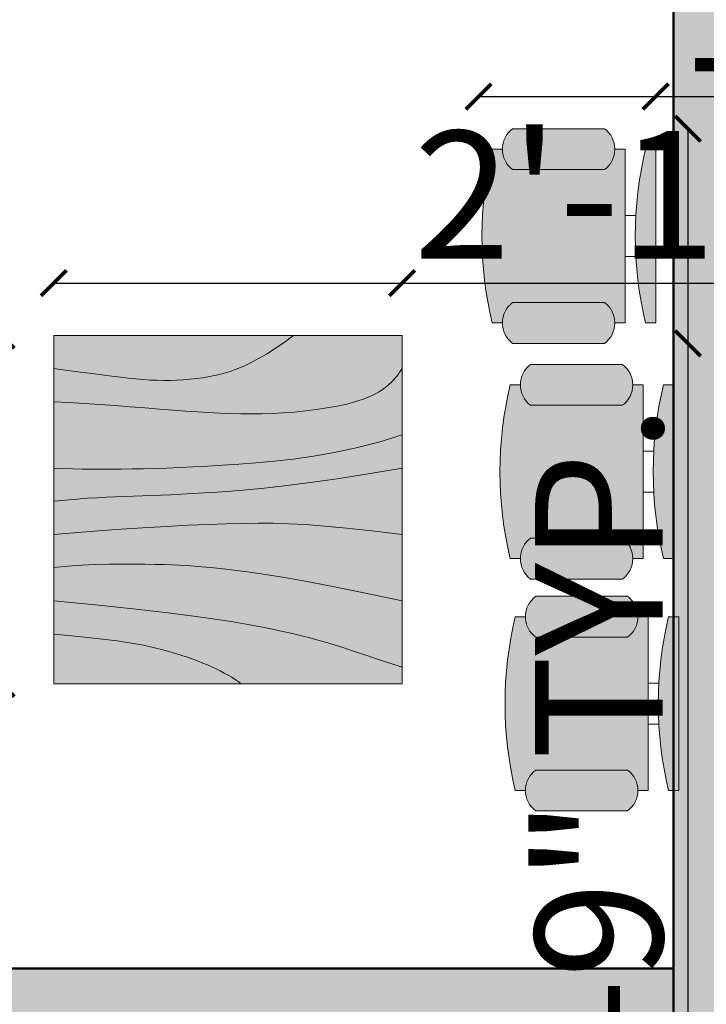
# Model space of a CAD drawing. Units: inches. Extents: x 2419 to 2878, y 1068 to 1713.
# Tile 10 of 20: x 2708 to 2775, y 1207 to 1304. Entities that reach past the tile are written whole.
import ezdxf

# ---------------------------------------------------------------- set-up
doc = ezdxf.new("R2010")
doc.units = ezdxf.units.IN
for name, color, linetype, lineweight in [('A-ANNO-DIMS', 2, 'Continuous', 18), ('A-FLOR-PRKG-PATT', 1, 'Continuous', 13), ('A-FURN', 8, 'Continuous', 18), ('A-FURN-PATT', 254, 'Continuous', 13), ('A-WALL', 7, 'Continuous', 50)]:
    doc.layers.add(name, color=color, linetype=linetype, lineweight=lineweight)
doc.layers.add('A-WALL-PATT', color=18, linetype='Continuous', lineweight=13, true_color=0x000000)
doc.styles.get("Standard").update_dxf_attribs({"font": 'arial.ttf'})
doc.dimstyles.new('ISO-25', dxfattribs={"dimtxt": 12.5, "dimasz": 2.5, "dimexe": 1.25, "dimexo": 0.625, "dimtad": 1, "dimdec": 0, "dimlunit": 4, "dimtxsty": 'Standard', "dimblk": 'ARCHTICK', "dimcen": 2.5, "dimse1": 1, "dimse2": 1, "dimclrd": 4, "dimadec": 0, "dimazin": 0, "dimtfac": 1, "dimtdec": 0, "dimtmove": 0, "dimatfit": 3, "dimfxl": 1, "dimarcsym": 0})

# ---------------------------------------------------------------- blocks, each defined once
blk = doc.blocks.new('Table - Square Woodgrain 42 x 42 in.')
blk.add_line((0, -42), (42, -42))
for points in [[(0, -4), (1.704, -4.2172), (3.2358, -4.4188), (4.615, -4.604), (5.8615, -4.7721), (6.9951, -4.9224), (8.0357, -5.0541), (9.0031, -5.1667), (9.9171, -5.2594), (10.7951, -5.3316), (11.6445, -5.3836), (12.4702, -5.4157), (13.277, -5.4283), (14.0698, -5.4217), (14.8535, -5.3964), (15.6331, -5.3526), (16.4133, -5.2908), (17.1986, -5.2103), (17.9913, -5.1062), (18.793, -4.9727), (19.6056, -4.8038), (20.4307, -4.5937), (21.2701, -4.3365), (22.1256, -4.0262), (22.9989, -3.6571), (23.888, -3.2272), (24.7756, -2.7516), (25.6408, -2.2491), (26.4624, -1.7387), (27.2195, -1.2395), (27.891, -0.7703), (28.456, -0.3501), (28.8934, 0.002)], [(0, -42), (0, 0), (42, 0), (42, -42)], [(0, -8), (1.8203, -8.1001), (3.6741, -8.2149), (5.5411, -8.3408), (7.4011, -8.4741), (9.2339, -8.6112), (11.0193, -8.7484), (12.7371, -8.8821), (14.3671, -9.0086), (15.8954, -9.1246), (17.3337, -9.2278), (18.6997, -9.3159), (20.0116, -9.387), (21.2871, -9.4389), (22.5442, -9.4696), (23.8008, -9.477), (25.0749, -9.459), (26.3791, -9.4137), (27.7049, -9.3403), (29.0383, -9.2382), (30.3655, -9.1068), (31.6728, -8.9455), (32.9461, -8.7535), (34.1717, -8.5304), (35.3358, -8.2756), (36.4268, -7.9863), (37.443, -7.6521), (38.3849, -7.2603), (39.253, -6.7986), (40.048, -6.2542), (40.7705, -5.6147), (41.421, -4.8674), (42, -4)], [(42, -12), (39.1784, -12.8621), (36.4519, -13.5654), (33.8246, -14.1294), (31.3004, -14.5731), (28.8832, -14.9161), (26.577, -15.1775), (24.3858, -15.3768), (22.3136, -15.5332), (20.3622, -15.6632), (18.5254, -15.7718), (16.7947, -15.8612), (15.1618, -15.9338), (13.6183, -15.9916), (12.1558, -16.0369), (10.7659, -16.0718), (9.4403, -16.0987), (8.1703, -16.1191), (6.9461, -16.1325), (5.7577, -16.1377), (4.595, -16.1335), (3.4479, -16.1188), (2.3064, -16.0924), (1.1604, -16.0532), (0, -16)], [(42, -16), (37.6529, -16.7365), (33.8802, -17.329), (30.6179, -17.7961), (27.8015, -18.1561), (25.3668, -18.4275), (23.2497, -18.6288), (21.3859, -18.7785), (19.7111, -18.8949), (18.1693, -18.9939), (16.7375, -19.0795), (15.401, -19.1534), (14.1449, -19.217), (12.9544, -19.2717), (11.8148, -19.3191), (10.7113, -19.3606), (9.6291, -19.3976), (8.5534, -19.4323), (7.47, -19.4689), (6.3643, -19.5122), (5.222, -19.5672), (4.0288, -19.6386), (2.7703, -19.7313), (1.4321, -19.8501), (0, -20)], [(0, -24), (3.9243, -23.6805), (7.4766, -23.4138), (10.6891, -23.1954), (13.5943, -23.0205), (16.2247, -22.8847), (18.6125, -22.7832), (20.7903, -22.7116), (22.7903, -22.6651), (24.6563, -22.642), (26.4764, -22.6507), (28.35, -22.7024), (30.3766, -22.8084), (32.6555, -22.98), (35.2861, -23.2283), (38.3678, -23.5645), (42, -24)], [(42, -32), (37.392, -31.017), (33.4585, -30.2231), (30.1291, -29.5949), (27.3334, -29.109), (25.0009, -28.742), (23.0612, -28.4707), (21.4439, -28.2716), (20.0786, -28.1215), (18.8998, -28.0002), (17.8609, -27.9014), (16.9206, -27.8219), (16.0371, -27.7588), (15.1691, -27.709), (14.2748, -27.6693), (13.3128, -27.6368), (12.2415, -27.6083), (11.0295, -27.5824), (9.6867, -27.5643), (8.233, -27.5608), (6.6884, -27.5787), (5.0728, -27.6248), (3.4062, -27.7058), (1.7086, -27.8286), (0, -28)], [(0, -32), (5.4026, -32.5358), (9.9494, -33.019), (13.7424, -33.4553), (16.8834, -33.8505), (19.4743, -34.2106), (21.6171, -34.5413), (23.4136, -34.8486), (24.9657, -35.1382), (26.3614, -35.4156), (27.6332, -35.6841), (28.7995, -35.9467), (29.8788, -36.2064), (30.8897, -36.4661), (31.8507, -36.7288), (32.7802, -36.9973), (33.6968, -37.2747), (34.6175, -37.5635), (35.5531, -37.8651), (36.5128, -38.1805), (37.506, -38.5108), (38.5421, -38.8568), (39.6302, -39.2197), (40.7797, -39.6004), (42, -40)], [(0, -36), (3.0098, -36.2857), (5.5354, -36.5643), (7.6368, -36.8359), (9.374, -37.1009), (10.807, -37.3597), (11.9957, -37.6126), (13.0002, -37.8599), (13.8804, -38.102), (14.6874, -38.3393), (15.4365, -38.5729), (16.1338, -38.8041), (16.7858, -39.0341), (17.3987, -39.264), (17.9787, -39.4952), (18.5322, -39.7288), (19.0655, -39.9662), (19.5832, -40.2081), (20.0842, -40.4544), (20.5657, -40.7046), (21.0249, -40.9581), (21.459, -41.2144), (21.8653, -41.4731), (22.2409, -41.7335), (22.5831, -41.9951)]]:
    blk.add_lwpolyline(points)
blk = doc.blocks.new('Chair - Desk')
for p, q in [((-8.5, 0), (-8.5, -1)), ((-8.5, 0), (8.5, 0)), ((8.5, 0), (8.5, -1)), ((-2, -3), (-2, -1.9355)), ((2, -1.9576), (2, -3)), ((-8.5, -3), (-8.5, -4)), ((-8.5, -3), (8.5, -3)), ((8.5, -3), (8.5, -4)), ((-10.5, -5), (-10.5, -14)), ((-6.5, -14), (-6.5, -5)), ((6.5, -5), (6.5, -14)), ((10.5, -14), (10.5, -5)), ((-8.5, -15), (-8.5, -16)), ((8.5, -15), (8.5, -16))]:
    blk.add_line(p, q)
for centre, radius, start, end in [((0, 34.625), 36.625, 256.5803, 283.4197), ((-8.5, -6.5), 2.5, 36.8699, 143.1301), ((8.5, -6.5), 2.5, 36.8699, 143.1301), ((-8.5, -12.5), 2.5, 216.8699, 323.1301), ((8.5, -12.5), 2.5, 216.8699, 323.1301), ((0, 19.625), 36.625, 256.5803, 283.4197)]:
    blk.add_arc(centre, radius, start, end)
blk = doc.blocks.new('_ArchTick')
at = {"color": 0, "linetype": 'ByBlock', "const_width": 0.15}
blk.add_lwpolyline([(-0.5, -0.5), (0.5, 0.5)], dxfattribs=at)
blk = doc.blocks.new('*D18')
at = {"layer": 'A-ANNO-DIMS', "color": 4, "lineweight": -2, "transparency": 16777216}
for p, q in [((2772.907, 1292.986), (2772.907, 1271.986)), ((2772.907, 1271.986), (2772.907, 1133.004))]:
    blk.add_line(p, q, dxfattribs=at)
at = {"layer": 'Defpoints', "color": 0, "transparency": 16777216}
for p in [(2769.757, 1292.986), (2769.757, 1271.986), (2772.907, 1271.986)]:
    blk.add_point(p, dxfattribs=at)
at = {"layer": 'A-ANNO-DIMS', "color": 4, "lineweight": -2, "transparency": 16777216, "xscale": 2.5, "yscale": 2.5, "zscale": 2.5}
for p, rotation in [((2772.907, 1292.986), 90), ((2772.907, 1271.986), 270)]:
    blk.add_blockref('_ArchTick', p, dxfattribs=dict(at, rotation=rotation))
at = {"layer": 'A-ANNO-DIMS', "color": 0, "transparency": 16777216, "insert": (2765.818, 1201.245), "char_height": 12.5, "attachment_point": 5, "rotation": 90}
blk.add_mtext('CHAIR 1\'-9" TYP.', dxfattribs=at)
blk = doc.blocks.new('*D19')
at = {"layer": 'A-ANNO-DIMS', "color": 4, "lineweight": -2, "transparency": 16777216}
for p, q in [((2752.423, 1296.136), (2769.757, 1296.136)), ((2769.757, 1296.136), (2877.651, 1296.136))]:
    blk.add_line(p, q, dxfattribs=at)
at = {"layer": 'Defpoints', "color": 0, "transparency": 16777216}
for p in [(2769.757, 1296.136), (2752.423, 1292.986), (2769.757, 1292.986)]:
    blk.add_point(p, dxfattribs=at)
at = {"layer": 'A-ANNO-DIMS', "color": 4, "lineweight": -2, "transparency": 16777216, "xscale": 2.5, "yscale": 2.5, "zscale": 2.5, "rotation": 180}
blk.add_blockref('_ArchTick', (2752.423, 1296.136), dxfattribs=at)
at = {"layer": 'A-ANNO-DIMS', "color": 4, "lineweight": -2, "transparency": 16777216, "xscale": 2.5, "yscale": 2.5, "zscale": 2.5}
blk.add_blockref('_ArchTick', (2769.757, 1296.136), dxfattribs=at)
at = {"layer": 'A-ANNO-DIMS', "color": 0, "transparency": 16777216, "insert": (2824.954, 1303.224), "char_height": 12.5, "attachment_point": 5}
blk.add_mtext('1\'-5 1/2" TYP.', dxfattribs=at)
blk = doc.blocks.new('*D32')
at = {"layer": 'A-ANNO-DIMS', "color": 4, "lineweight": -2, "transparency": 16777216}
for p, q in [((2705.74, 1272.772), (2705.74, 1458.173)), ((2705.74, 1238.68), (2705.74, 1272.772))]:
    blk.add_line(p, q, dxfattribs=at)
at = {"layer": 'Defpoints', "color": 0, "transparency": 16777216}
for p in [(2705.74, 1272.772), (2710.853, 1272.772), (2710.853, 1238.68)]:
    blk.add_point(p, dxfattribs=at)
at = {"layer": 'A-ANNO-DIMS', "color": 4, "lineweight": -2, "transparency": 16777216, "xscale": 2.5, "yscale": 2.5, "zscale": 2.5}
for p, rotation in [((2705.74, 1272.772), 90), ((2705.74, 1238.68), 270)]:
    blk.add_blockref('_ArchTick', p, dxfattribs=dict(at, rotation=rotation))
at = {"layer": 'A-ANNO-DIMS', "color": 0, "transparency": 16777216, "insert": (2698.268, 1366.722), "char_height": 12.5, "attachment_point": 5, "rotation": 90}
blk.add_mtext('SQUARE TABLE 2\'-10"', dxfattribs=at)
blk = doc.blocks.new('*D33')
at = {"layer": 'A-ANNO-DIMS', "color": 4, "lineweight": -2, "transparency": 16777216}
for p, q in [((2710.853, 1277.886), (2744.943, 1277.886)), ((2744.943, 1277.886), (2791.847, 1277.886))]:
    blk.add_line(p, q, dxfattribs=at)
at = {"layer": 'Defpoints', "color": 0, "transparency": 16777216}
for p in [(2744.943, 1277.886), (2710.853, 1272.772), (2744.943, 1272.772)]:
    blk.add_point(p, dxfattribs=at)
at = {"layer": 'A-ANNO-DIMS', "color": 4, "lineweight": -2, "transparency": 16777216, "xscale": 2.5, "yscale": 2.5, "zscale": 2.5, "rotation": 180}
blk.add_blockref('_ArchTick', (2710.853, 1277.886), dxfattribs=at)
at = {"layer": 'A-ANNO-DIMS', "color": 4, "lineweight": -2, "transparency": 16777216, "xscale": 2.5, "yscale": 2.5, "zscale": 2.5}
blk.add_blockref('_ArchTick', (2744.943, 1277.886), dxfattribs=at)
at = {"layer": 'A-ANNO-DIMS', "color": 0, "transparency": 16777216, "insert": (2769.645, 1284.893), "char_height": 12.5, "attachment_point": 5}
blk.add_mtext('2\'-10"', dxfattribs=at)
blk = doc.blocks.new('*D36')
at = {"layer": 'A-ANNO-DIMS', "color": 4, "lineweight": -2, "transparency": 16777216}
blk.add_line((2656.741, 1605.013), (2736.32, 1605.013), dxfattribs=at)
at = {"layer": 'Defpoints', "color": 0, "transparency": 16777216}
for p in [(2736.32, 1605.013), (2656.741, 1205.813), (2736.32, 1205.813)]:
    blk.add_point(p, dxfattribs=at)
at = {"layer": 'A-ANNO-DIMS', "color": 4, "lineweight": -2, "transparency": 16777216, "xscale": 2.5, "yscale": 2.5, "zscale": 2.5, "rotation": 180}
blk.add_blockref('_ArchTick', (2656.741, 1605.013), dxfattribs=at)
at = {"layer": 'A-ANNO-DIMS', "color": 4, "lineweight": -2, "transparency": 16777216, "xscale": 2.5, "yscale": 2.5, "zscale": 2.5}
blk.add_blockref('_ArchTick', (2736.32, 1605.013), dxfattribs=at)
at = {"layer": 'A-ANNO-DIMS', "color": 0, "transparency": 16777216, "insert": (2696.531, 1612.101), "char_height": 12.5, "attachment_point": 5}
blk.add_mtext('6\'-7 1/2"', dxfattribs=at)
blk = doc.blocks.new('*D37')
at = {"layer": 'A-ANNO-DIMS', "color": 4, "lineweight": -2, "transparency": 16777216}
for p, q in [((2736.32, 1605.013), (2771.514, 1605.013)), ((2771.514, 1605.013), (2818.418, 1605.013))]:
    blk.add_line(p, q, dxfattribs=at)
at = {"layer": 'Defpoints', "color": 0, "transparency": 16777216}
for p in [(2771.514, 1605.013), (2736.32, 1205.813), (2771.514, 1205.813)]:
    blk.add_point(p, dxfattribs=at)
at = {"layer": 'A-ANNO-DIMS', "color": 4, "lineweight": -2, "transparency": 16777216, "xscale": 2.5, "yscale": 2.5, "zscale": 2.5, "rotation": 180}
blk.add_blockref('_ArchTick', (2736.32, 1605.013), dxfattribs=at)
at = {"layer": 'A-ANNO-DIMS', "color": 4, "lineweight": -2, "transparency": 16777216, "xscale": 2.5, "yscale": 2.5, "zscale": 2.5}
blk.add_blockref('_ArchTick', (2771.514, 1605.013), dxfattribs=at)
at = {"layer": 'A-ANNO-DIMS', "color": 0, "transparency": 16777216, "insert": (2796.216, 1611.914), "char_height": 12.5, "attachment_point": 5}
blk.add_mtext('2\'-11"', dxfattribs=at)
blk = doc.blocks.new('*D40')
at = {"layer": 'A-ANNO-DIMS', "color": 4, "lineweight": -2, "transparency": 16777216}
for p, q in [((2858.714, 1205.813), (2858.714, 1281.843)), ((2858.714, 1171.283), (2858.714, 1205.813))]:
    blk.add_line(p, q, dxfattribs=at)
at = {"layer": 'Defpoints', "color": 0, "transparency": 16777216}
for p in [(2736.32, 1205.813), (2858.714, 1205.813), (2736.32, 1171.283)]:
    blk.add_point(p, dxfattribs=at)
at = {"layer": 'A-ANNO-DIMS', "color": 4, "lineweight": -2, "transparency": 16777216, "xscale": 2.5, "yscale": 2.5, "zscale": 2.5}
for p, rotation in [((2858.714, 1205.813), 90), ((2858.714, 1171.283), 270)]:
    blk.add_blockref('_ArchTick', p, dxfattribs=dict(at, rotation=rotation))
at = {"layer": 'A-ANNO-DIMS', "color": 0, "transparency": 16777216, "insert": (2851.626, 1245.078), "char_height": 12.5, "attachment_point": 5, "rotation": 90}
blk.add_mtext('2\'-10 1/2"', dxfattribs=at)
blk = doc.blocks.new('*D51')
at = {"layer": 'A-ANNO-DIMS', "color": 4, "lineweight": -2, "transparency": 16777216}
for p, q in [((2738.514, 1079.925), (2771.514, 1079.925)), ((2771.514, 1079.925), (2808.706, 1079.925))]:
    blk.add_line(p, q, dxfattribs=at)
at = {"layer": 'Defpoints', "color": 0, "transparency": 16777216}
for p in [(2738.514, 1447.891), (2771.514, 1437.391), (2771.514, 1079.925)]:
    blk.add_point(p, dxfattribs=at)
at = {"layer": 'A-ANNO-DIMS', "color": 4, "lineweight": -2, "transparency": 16777216, "xscale": 2.5, "yscale": 2.5, "zscale": 2.5, "rotation": 180}
blk.add_blockref('_ArchTick', (2738.514, 1079.925), dxfattribs=at)
at = {"layer": 'A-ANNO-DIMS', "color": 4, "lineweight": -2, "transparency": 16777216, "xscale": 2.5, "yscale": 2.5, "zscale": 2.5}
blk.add_blockref('_ArchTick', (2771.514, 1079.925), dxfattribs=at)
at = {"layer": 'A-ANNO-DIMS', "color": 0, "transparency": 16777216, "insert": (2791.36, 1086.932), "char_height": 12.5, "attachment_point": 5}
blk.add_mtext('2\'-9"', dxfattribs=at)
blk = doc.blocks.new('*D53')
at = {"layer": 'A-ANNO-DIMS', "color": 4, "lineweight": -2, "transparency": 16777216}
for p, q in [((2638.792, 1605.013), (2667.311, 1605.013)), ((2667.311, 1605.013), (2733.629, 1605.013))]:
    blk.add_line(p, q, dxfattribs=at)
at = {"layer": 'Defpoints', "color": 0, "transparency": 16777216}
for p in [(2667.311, 1605.013), (2638.792, 1217.382), (2667.311, 1217.382)]:
    blk.add_point(p, dxfattribs=at)
at = {"layer": 'A-ANNO-DIMS', "color": 4, "lineweight": -2, "transparency": 16777216, "xscale": 2.5, "yscale": 2.5, "zscale": 2.5, "rotation": 180}
blk.add_blockref('_ArchTick', (2638.792, 1605.013), dxfattribs=at)
at = {"layer": 'A-ANNO-DIMS', "color": 4, "lineweight": -2, "transparency": 16777216, "xscale": 2.5, "yscale": 2.5, "zscale": 2.5}
blk.add_blockref('_ArchTick', (2667.311, 1605.013), dxfattribs=at)
at = {"layer": 'A-ANNO-DIMS', "color": 0, "transparency": 16777216, "insert": (2701.72, 1612.101), "char_height": 12.5, "attachment_point": 5}
blk.add_mtext('2\'-4 1/2"', dxfattribs=at)
blk = doc.blocks.new('*D61')
at = {"layer": 'A-ANNO-DIMS', "color": 4, "lineweight": -2, "transparency": 16777216}
blk.add_line((2730.514, 1079.925), (2771.514, 1079.925), dxfattribs=at)
at = {"layer": 'Defpoints', "color": 0, "transparency": 16777216}
for p in [(2730.514, 1414.813), (2771.514, 1414.813), (2771.514, 1079.925)]:
    blk.add_point(p, dxfattribs=at)
at = {"layer": 'A-ANNO-DIMS', "color": 4, "lineweight": -2, "transparency": 16777216, "xscale": 2.5, "yscale": 2.5, "zscale": 2.5, "rotation": 180}
blk.add_blockref('_ArchTick', (2730.514, 1079.925), dxfattribs=at)
at = {"layer": 'A-ANNO-DIMS', "color": 4, "lineweight": -2, "transparency": 16777216, "xscale": 2.5, "yscale": 2.5, "zscale": 2.5}
blk.add_blockref('_ArchTick', (2771.514, 1079.925), dxfattribs=at)
at = {"layer": 'A-ANNO-DIMS', "color": 0, "transparency": 16777216, "insert": (2751.014, 1086.936), "char_height": 12.5, "attachment_point": 5}
blk.add_mtext('3\'-5"', dxfattribs=at)

msp = doc.modelspace()

# ---------------------------------------------------------------- hatches: boundary and pattern name
at = {"layer": 'A-FLOR-PRKG-PATT'}
h = msp.add_hatch(color=256, dxfattribs=at)
h.dxf.hatch_style = 1
edge = h.paths.add_edge_path()
edge.add_ellipse((2561.374, 1279.453), major_axis=(3.988, 0), ratio=0.842304, start_angle=0.64655, end_angle=90)
edge.add_line((2561.374, 1282.813), (2511.571, 1282.813))
edge.add_ellipse((2511.571, 1279.453), major_axis=(3.988, 0), ratio=0.842304, start_angle=90, end_angle=179.35345)
edge.add_ellipse((10560.892, 1188.617), major_axis=(-8054.031, 0), ratio=0.84230387, start_angle=-0.6465541, end_angle=-0.6282372)
edge.add_ellipse((2509.23, 1276.906), major_axis=(1.687, 0), ratio=0.842304, start_angle=179.37176, end_angle=248.46476)
edge.add_ellipse((10560.329, 1188.617), major_axis=(8052.293, 0), ratio=0.84230387, start_angle=179.3534459, end_angle=179.3813568, ccw=False)
edge.add_ellipse((2511.008, 1279.453), major_axis=(2.25, 0), ratio=0.842304, start_angle=90, end_angle=179.35345, ccw=False)
edge.add_line((2511.008, 1281.348), (2561.936, 1281.348))
edge.add_ellipse((2561.936, 1279.453), major_axis=(-2.25, 0), ratio=0.842304, start_angle=180.64655, end_angle=270, ccw=False)
edge.add_ellipse((-5487.385, 1188.617), major_axis=(8052.293, 0), ratio=0.84230387, start_angle=0.5282715, end_angle=0.6465541, ccw=False)
edge.add_ellipse((2563.715, 1276.906), major_axis=(-1.687, 0), ratio=0.842304, start_angle=111.53524, end_angle=180.62824)
edge.add_ellipse((-5487.947, 1188.617), major_axis=(-8054.031, 0), ratio=0.84230387, start_angle=180.6282372, end_angle=180.6465541)
edge = h.paths.add_edge_path()
edge.add_ellipse((2564.908, 1261.91), major_axis=(-1.125, 0), ratio=0.842304, start_angle=180, end_angle=270)
edge.add_line((2564.908, 1262.857), (2564.426, 1262.857))
edge.add_ellipse((-5487.385, 1188.617), major_axis=(8052.293, 0), ratio=0.84230387, start_angle=0.3838668, end_angle=0.5282715, ccw=False)
edge.add_line((2564.654, 1242.564), (2564.908, 1242.564))
edge.add_ellipse((2564.908, 1243.512), major_axis=(-1.125, 0), ratio=0.842304, start_angle=90, end_angle=180)
edge.add_line((2566.033, 1243.512), (2566.033, 1261.91))
edge = h.paths.add_edge_path()
edge.add_ellipse((2564.908, 1174.989), major_axis=(1.125, 0), ratio=0.842304, start_angle=0, end_angle=90)
edge.add_line((2564.908, 1175.936), (2564.894, 1175.936))
edge.add_ellipse((-5487.385, 1188.617), major_axis=(8052.293, 0), ratio=0.84230387, start_angle=-0.1349866, end_angle=-0.0902291, ccw=False)
edge.add_ellipse((2163.343, 1170.913), major_axis=(401.537, 0), ratio=0.8423039, start_angle=-2.17995, end_angle=-0.13561, ccw=False)
edge.add_line((2564.47, 1155.643), (2564.908, 1155.643))
edge.add_ellipse((2564.908, 1156.591), major_axis=(-1.125, 0), ratio=0.842304, start_angle=90, end_angle=180)
edge.add_line((2566.033, 1156.591), (2566.033, 1174.989))
h.paths.add_polyline_path([(2574.476, 1207.448), (2633.94, 1207.448), (2633.94, 1217.366), (2574.476, 1217.366)], flags=9)
h.paths.add_polyline_path([(2574.454, 1217.828), (2610.472, 1217.828), (2610.472, 1227.879), (2574.454, 1227.879)], flags=9)
h.paths.add_polyline_path([(2672.426, 1304.02), (2718.617, 1304.02), (2718.617, 1313.939), (2672.426, 1313.939)], flags=9)
h.paths.add_polyline_path([(2672.404, 1314.4), (2750.128, 1314.4), (2750.128, 1324.451), (2672.404, 1324.451)], flags=9)
h.paths.add_polyline_path([(2500.432, 1374.444), (2544.803, 1374.444), (2544.803, 1384.362), (2500.432, 1384.362)], flags=9)
h.paths.add_polyline_path([(2500.41, 1384.824), (2566.075, 1384.824), (2566.075, 1394.875), (2500.41, 1394.875)], flags=9)
h.paths.add_polyline_path([(2738.933, 1376.749), (2778.273, 1376.749), (2778.273, 1386.667), (2738.933, 1386.667)], flags=9)
h.paths.add_polyline_path([(2659.12, 1357.8), (2703.492, 1357.8), (2703.492, 1367.718), (2659.12, 1367.718)], flags=9)
h.paths.add_polyline_path([(2659.098, 1368.18), (2694.114, 1368.18), (2694.114, 1378.23), (2659.098, 1378.23)], flags=9)
h.paths.add_polyline_path([(2730.123, 1466.067), (2769.463, 1466.067), (2769.463, 1475.986), (2730.123, 1475.986)], flags=9)
h.paths.add_polyline_path([(2730.101, 1476.447), (2765.117, 1476.447), (2765.117, 1486.498), (2730.101, 1486.498)], flags=9)
h.paths.add_polyline_path([(2730.382, 1518.647), (2761.48, 1518.647), (2761.48, 1528.566), (2730.382, 1528.566)], flags=9)
h.paths.add_polyline_path([(2730.361, 1529.028), (2780.958, 1529.028), (2780.958, 1539.072), (2730.361, 1539.072)], flags=9)
h.paths.add_polyline_path([(2629.32, 1455.189), (2688.784, 1455.189), (2688.784, 1465.107), (2629.32, 1465.107)], flags=9)
h.paths.add_polyline_path([(2629.298, 1465.569), (2681.902, 1465.569), (2681.902, 1475.62), (2629.298, 1475.62)], flags=9)
h.paths.add_polyline_path([(2513.229, 1456.484), (2562.631, 1456.484), (2562.631, 1466.402), (2513.229, 1466.402)], flags=9)
h.paths.add_polyline_path([(2513.208, 1466.865), (2556.26, 1466.865), (2556.26, 1476.909), (2513.208, 1476.909)], flags=9)
h.paths.add_polyline_path([(2488.87, 1521.538), (2519.968, 1521.538), (2519.968, 1531.456), (2488.87, 1531.456)], flags=9)
h.paths.add_polyline_path([(2536.549, 1543.507), (2580.923, 1543.507), (2580.923, 1553.432), (2536.549, 1553.432)], flags=9)
h.paths.add_polyline_path([(2536.557, 1553.921), (2573.525, 1553.921), (2573.525, 1563.8), (2536.557, 1563.8)], flags=9)
at = {"layer": 'A-FURN-PATT'}
h = msp.add_hatch(color=256, dxfattribs=at)
h.dxf.hatch_style = 1
h.paths.add_polyline_path([(2768.514, 1267.928), (2767.514, 1267.928, -0.236068), (2766.514, 1265.928), (2757.514, 1265.928, -0.236068), (2756.514, 1267.928), (2755.514, 1267.928, 0.117647), (2755.514, 1250.928), (2756.514, 1250.928, -0.236068), (2757.514, 1252.928), (2766.514, 1252.928, -0.236068), (2767.514, 1250.928), (2768.514, 1250.928)])
h.paths.add_polyline_path([(2766.757, 1290.986), (2765.757, 1290.986, -0.236068), (2764.757, 1288.986), (2755.757, 1288.986, -0.236068), (2754.757, 1290.986), (2753.757, 1290.986, 0.117647), (2753.757, 1273.986), (2754.757, 1273.986, -0.236068), (2755.757, 1275.986), (2764.757, 1275.986, -0.236068), (2765.757, 1273.986), (2766.757, 1273.986)])
h.paths.add_polyline_path([(2769.013, 1245.244), (2768.013, 1245.244, -0.236068), (2767.013, 1243.244), (2758.013, 1243.244, -0.236068), (2757.013, 1245.244), (2756.013, 1245.244, 0.117647), (2756.013, 1228.244), (2757.013, 1228.244, -0.236068), (2758.013, 1230.244), (2767.013, 1230.244, -0.236068), (2768.013, 1228.244), (2769.013, 1228.244)])
h.paths.add_polyline_path([(2764.757, 1275.986), (2755.757, 1275.986, 0.236068), (2754.757, 1273.986, 0.236068), (2755.757, 1271.986), (2764.757, 1271.986, 0.5)])
h.paths.add_polyline_path([(2764.757, 1292.986), (2755.757, 1292.986, 0.5), (2755.757, 1288.986), (2764.757, 1288.986, 0.5)])
h.paths.add_polyline_path([(2766.514, 1269.928), (2757.514, 1269.928, 0.5), (2757.514, 1265.928), (2766.514, 1265.928, 0.5)])
h.paths.add_polyline_path([(2767.013, 1247.244), (2758.013, 1247.244, 0.5), (2758.013, 1243.244), (2767.013, 1243.244, 0.5)])
h.paths.add_polyline_path([(2766.514, 1252.928), (2757.514, 1252.928, 0.236068), (2756.514, 1250.928, 0.236068), (2757.514, 1248.928), (2766.514, 1248.928, 0.5)])
h.paths.add_polyline_path([(2767.013, 1230.244), (2758.013, 1230.244, 0.236068), (2757.013, 1228.244, 0.236068), (2758.013, 1226.244), (2767.013, 1226.244, 0.5)])
h.paths.add_polyline_path([(2771.514, 1267.928), (2770.514, 1267.928, 0.117647), (2770.514, 1250.928), (2771.514, 1250.928)])
h.paths.add_polyline_path([(2769.757, 1290.986), (2768.757, 1290.986, 0.117647), (2768.757, 1273.986), (2769.757, 1273.986)])
h.paths.add_polyline_path([(2771.514, 1245.244), (2771.013, 1245.244, 0.117647), (2771.013, 1228.244), (2771.514, 1228.244)])
h = msp.add_hatch(color=256, dxfattribs=at)
h.dxf.hatch_style = 1
h.paths.add_polyline_path([(2730.243, 1270.151), (2730.963, 1270.537), (2731.665, 1270.945), (2732.332, 1271.359), (2732.947, 1271.764), (2733.492, 1272.145), (2733.95, 1272.486), (2734.303, 1272.77), (2710.853, 1272.77), (2710.853, 1269.524), (2712.237, 1269.347), (2713.48, 1269.184), (2714.599, 1269.033), (2715.611, 1268.897), (2716.531, 1268.775), (2717.376, 1268.668), (2718.161, 1268.577), (2718.903, 1268.501), (2719.615, 1268.443), (2720.305, 1268.401), (2720.975, 1268.375), (2721.63, 1268.364), (2722.273, 1268.37), (2722.91, 1268.39), (2723.542, 1268.426), (2724.176, 1268.476), (2724.813, 1268.541), (2725.456, 1268.626), (2726.107, 1268.734), (2726.767, 1268.871), (2727.436, 1269.042), (2728.118, 1269.251), (2728.812, 1269.502), (2729.521, 1269.802)], flags=17)
h.paths.add_polyline_path([(2738.589, 1265.846), (2739.534, 1266.053), (2740.42, 1266.288), (2741.245, 1266.559), (2742.009, 1266.877), (2742.714, 1267.252), (2743.359, 1267.694), (2743.946, 1268.213), (2744.474, 1268.82), (2744.943, 1269.524), (2744.943, 1272.77), (2734.303, 1272.77), (2733.95, 1272.486), (2733.492, 1272.145), (2732.947, 1271.764), (2732.332, 1271.359), (2731.665, 1270.945), (2730.963, 1270.537), (2730.243, 1270.151), (2729.521, 1269.802), (2728.812, 1269.502), (2728.118, 1269.251), (2727.436, 1269.042), (2726.767, 1268.871), (2726.107, 1268.734), (2725.456, 1268.626), (2724.813, 1268.541), (2724.176, 1268.476), (2723.542, 1268.426), (2722.91, 1268.39), (2722.273, 1268.37), (2721.63, 1268.364), (2720.975, 1268.375), (2720.305, 1268.401), (2719.615, 1268.443), (2718.903, 1268.501), (2718.161, 1268.577), (2717.376, 1268.668), (2716.531, 1268.775), (2715.611, 1268.897), (2714.599, 1269.033), (2713.48, 1269.184), (2712.237, 1269.347), (2710.853, 1269.524), (2710.853, 1266.277), (2712.331, 1266.196), (2713.836, 1266.103), (2715.351, 1266), (2716.861, 1265.892), (2718.348, 1265.781), (2719.797, 1265.67), (2721.192, 1265.561), (2722.515, 1265.458), (2723.755, 1265.364), (2724.923, 1265.28), (2726.031, 1265.209), (2727.096, 1265.151), (2728.131, 1265.109), (2729.152, 1265.084), (2730.172, 1265.078), (2731.206, 1265.093), (2732.265, 1265.13), (2733.341, 1265.189), (2734.423, 1265.272), (2735.5, 1265.379), (2736.561, 1265.51), (2737.595, 1265.665)])
h.paths.add_polyline_path([(2740.44, 1261.76), (2742.653, 1262.331), (2744.943, 1263.03), (2744.943, 1269.524), (2744.474, 1268.82), (2743.946, 1268.213), (2743.359, 1267.694), (2742.714, 1267.252), (2742.009, 1266.877), (2741.245, 1266.559), (2740.42, 1266.288), (2739.534, 1266.053), (2738.589, 1265.846), (2737.595, 1265.665), (2736.561, 1265.51), (2735.5, 1265.379), (2734.423, 1265.272), (2733.341, 1265.189), (2732.265, 1265.13), (2731.206, 1265.093), (2730.172, 1265.078), (2729.152, 1265.084), (2728.131, 1265.109), (2727.096, 1265.151), (2726.031, 1265.209), (2724.923, 1265.28), (2723.755, 1265.364), (2722.515, 1265.458), (2721.192, 1265.561), (2719.797, 1265.67), (2718.348, 1265.781), (2716.861, 1265.892), (2715.351, 1266), (2713.836, 1266.103), (2712.331, 1266.196), (2710.853, 1266.277), (2710.853, 1259.784), (2711.795, 1259.74), (2712.725, 1259.709), (2713.652, 1259.687), (2714.583, 1259.675), (2715.527, 1259.672), (2716.491, 1259.676), (2717.485, 1259.687), (2718.516, 1259.704), (2719.592, 1259.725), (2720.72, 1259.754), (2721.907, 1259.79), (2723.16, 1259.837), (2724.485, 1259.896), (2725.89, 1259.969), (2727.381, 1260.057), (2728.965, 1260.163), (2730.647, 1260.289), (2732.425, 1260.451), (2734.297, 1260.663), (2736.259, 1260.942), (2738.308, 1261.302)])
h.paths.add_polyline_path([(2741.995, 1253.644), (2739.494, 1253.917), (2737.359, 1254.118), (2735.509, 1254.257), (2733.864, 1254.344), (2732.343, 1254.385), (2730.866, 1254.393), (2729.352, 1254.374), (2727.728, 1254.336), (2725.961, 1254.278), (2724.023, 1254.196), (2721.888, 1254.085), (2719.529, 1253.943), (2716.922, 1253.766), (2714.039, 1253.55), (2710.853, 1253.29), (2710.853, 1250.044), (2712.24, 1250.183), (2713.618, 1250.282), (2714.971, 1250.348), (2716.282, 1250.386), (2717.536, 1250.4), (2718.716, 1250.397), (2719.806, 1250.383), (2720.789, 1250.362), (2721.659, 1250.338), (2722.44, 1250.312), (2723.166, 1250.28), (2723.87, 1250.239), (2724.587, 1250.188), (2725.351, 1250.124), (2726.194, 1250.043), (2727.151, 1249.945), (2728.259, 1249.823), (2729.571, 1249.662), (2731.146, 1249.441), (2733.039, 1249.143), (2735.308, 1248.749), (2738.011, 1248.239), (2741.203, 1247.595), (2744.943, 1246.797), (2744.943, 1253.29)])
h.paths.add_polyline_path([(2744.943, 1259.784), (2741.415, 1259.186), (2738.353, 1258.705), (2735.705, 1258.326), (2733.419, 1258.034), (2731.443, 1257.813), (2729.724, 1257.65), (2728.212, 1257.528), (2726.852, 1257.434), (2725.601, 1257.354), (2724.439, 1257.284), (2723.354, 1257.224), (2722.334, 1257.173), (2721.368, 1257.128), (2720.443, 1257.09), (2719.547, 1257.056), (2718.669, 1257.026), (2717.796, 1256.998), (2716.917, 1256.968), (2716.019, 1256.933), (2715.092, 1256.888), (2714.124, 1256.83), (2713.102, 1256.755), (2712.016, 1256.659), (2710.853, 1256.537), (2710.853, 1253.29), (2714.039, 1253.55), (2716.922, 1253.766), (2719.529, 1253.943), (2721.888, 1254.085), (2724.023, 1254.196), (2725.961, 1254.278), (2727.728, 1254.336), (2729.352, 1254.374), (2730.866, 1254.393), (2732.343, 1254.385), (2733.864, 1254.344), (2735.509, 1254.257), (2737.359, 1254.118), (2739.494, 1253.917), (2741.995, 1253.644), (2744.943, 1253.29)])
h.paths.add_polyline_path([(2726.328, 1240.331), (2725.895, 1240.524), (2725.446, 1240.713), (2724.975, 1240.901), (2724.478, 1241.088), (2723.949, 1241.274), (2723.383, 1241.462), (2722.775, 1241.652), (2722.12, 1241.844), (2721.405, 1242.041), (2720.59, 1242.241), (2719.625, 1242.447), (2718.462, 1242.657), (2717.052, 1242.872), (2715.346, 1243.092), (2713.296, 1243.318), (2710.853, 1243.55), (2710.853, 1238.68), (2729.189, 1238.68), (2728.906, 1238.897), (2728.601, 1239.108), (2728.271, 1239.318), (2727.919, 1239.526), (2727.546, 1239.732), (2727.155, 1239.935), (2726.749, 1240.135)], flags=17)
h.paths.add_polyline_path([(2731.117, 1244.25), (2729.858, 1244.485), (2728.399, 1244.734), (2726.66, 1245.003), (2724.557, 1245.295), (2722.008, 1245.616), (2718.929, 1245.97), (2715.239, 1246.362), (2710.853, 1246.797), (2710.853, 1243.55), (2713.296, 1243.318), (2715.346, 1243.092), (2717.052, 1242.872), (2718.462, 1242.657), (2719.625, 1242.447), (2720.59, 1242.241), (2721.405, 1242.041), (2722.12, 1241.844), (2722.775, 1241.652), (2723.383, 1241.462), (2723.949, 1241.274), (2724.478, 1241.088), (2724.975, 1240.901), (2725.446, 1240.713), (2725.895, 1240.524), (2726.328, 1240.331), (2726.749, 1240.135), (2727.155, 1239.935), (2727.546, 1239.732), (2727.919, 1239.526), (2728.271, 1239.318), (2728.601, 1239.108), (2728.906, 1238.897), (2729.189, 1238.68), (2744.943, 1238.68), (2744.943, 1240.304), (2743.953, 1240.628), (2743.02, 1240.937), (2742.137, 1241.232), (2741.296, 1241.512), (2740.49, 1241.78), (2739.711, 1242.036), (2738.951, 1242.281), (2738.204, 1242.516), (2737.46, 1242.741), (2736.706, 1242.959), (2735.926, 1243.172), (2735.105, 1243.383), (2734.229, 1243.594), (2733.282, 1243.807), (2732.25, 1244.025)])
h.paths.add_polyline_path([(2741.203, 1247.595), (2738.011, 1248.239), (2735.308, 1248.749), (2733.039, 1249.143), (2731.146, 1249.441), (2729.571, 1249.662), (2728.259, 1249.823), (2727.151, 1249.945), (2726.194, 1250.043), (2725.351, 1250.124), (2724.587, 1250.188), (2723.87, 1250.239), (2723.166, 1250.28), (2722.44, 1250.312), (2721.659, 1250.338), (2720.789, 1250.362), (2719.806, 1250.383), (2718.716, 1250.397), (2717.536, 1250.4), (2716.282, 1250.386), (2714.971, 1250.348), (2713.618, 1250.282), (2712.24, 1250.183), (2710.853, 1250.044), (2710.853, 1246.797), (2715.239, 1246.362), (2718.929, 1245.97), (2722.008, 1245.616), (2724.557, 1245.295), (2726.66, 1245.003), (2728.399, 1244.734), (2729.858, 1244.485), (2731.117, 1244.25), (2732.25, 1244.025), (2733.282, 1243.807), (2734.229, 1243.594), (2735.105, 1243.383), (2735.926, 1243.172), (2736.706, 1242.959), (2737.46, 1242.741), (2738.204, 1242.516), (2738.951, 1242.281), (2739.711, 1242.036), (2740.49, 1241.78), (2741.296, 1241.512), (2742.137, 1241.232), (2743.02, 1240.937), (2743.953, 1240.628), (2744.943, 1240.304), (2744.943, 1246.797)])
h.paths.add_polyline_path([(2733.419, 1258.034), (2735.705, 1258.326), (2738.353, 1258.705), (2741.415, 1259.186), (2744.943, 1259.784), (2744.943, 1263.03), (2742.653, 1262.331), (2740.44, 1261.76), (2738.308, 1261.302), (2736.259, 1260.942), (2734.297, 1260.663), (2732.425, 1260.451), (2730.647, 1260.289), (2728.965, 1260.163), (2727.381, 1260.057), (2725.89, 1259.969), (2724.485, 1259.896), (2723.16, 1259.837), (2721.907, 1259.79), (2720.72, 1259.754), (2719.592, 1259.725), (2718.516, 1259.704), (2717.485, 1259.687), (2716.491, 1259.676), (2715.527, 1259.672), (2714.583, 1259.675), (2713.652, 1259.687), (2712.725, 1259.709), (2711.795, 1259.74), (2710.853, 1259.784), (2710.853, 1256.537), (2712.016, 1256.659), (2713.102, 1256.755), (2714.124, 1256.83), (2715.092, 1256.888), (2716.019, 1256.933), (2716.917, 1256.968), (2717.796, 1256.998), (2718.669, 1257.026), (2719.547, 1257.056), (2720.443, 1257.09), (2721.368, 1257.128), (2722.334, 1257.173), (2723.354, 1257.224), (2724.439, 1257.284), (2725.601, 1257.354), (2726.852, 1257.434), (2728.212, 1257.528), (2729.724, 1257.65), (2731.443, 1257.813)])
at = {"layer": 'A-WALL-PATT'}
h = msp.add_hatch(color=256, dxfattribs=at)
h.dxf.hatch_style = 1
h.paths.add_polyline_path([(2780.514, 1577.813), (2471.514, 1577.813), (2471.514, 1121.813), (2780.514, 1121.813)])
h.paths.add_polyline_path([(2480.514, 1568.813), (2771.514, 1568.813), (2771.514, 1130.813), (2480.514, 1130.813)], flags=16)
h.paths.add_polyline_path([(2528.514, 1568.813), (2528.514, 1512.813), (2594.514, 1512.813), (2594.514, 1414.813), (2596.568, 1414.813), (2596.568, 1441.609), (2597.816, 1441.609), (2597.816, 1441.582, -0.384016), (2625.035, 1414.813), (2725.514, 1414.813), (2725.514, 1567.545), (2728.302, 1567.545), (2746.887, 1567.545), (2746.887, 1566.732), (2746.87, 1566.732, -0.367216), (2730.514, 1549.092), (2730.514, 1512.813), (2750.853, 1512.813), (2750.853, 1510.025, -0.401453), (2733.081, 1491.458), (2733.081, 1491.44), (2732.268, 1491.44), (2732.268, 1507.813), (2730.514, 1507.813), (2730.514, 1408.813), (2736.514, 1408.813), (2736.514, 1349.813), (2632.514, 1349.813), (2632.514, 1408.813), (2528.514, 1408.813), (2528.514, 1414.813), (2503.967, 1414.813), (2503.967, 1494.852), (2558.379, 1494.852), (2558.379, 1507.813), (2529.965, 1507.813, -0.414214), (2530.821, 1506.957), (2530.821, 1497.257, -0.414214), (2529.965, 1496.401), (2514.559, 1496.401, -0.414214), (2513.703, 1497.257), (2513.703, 1506.957, -0.414214), (2514.559, 1507.813), (2528.514, 1507.813), (2528.514, 1512.813), (2480.514, 1512.813)], flags=0)
h.paths.add_polyline_path([(2516.262, 1507.813), (2528.262, 1507.813), (2528.262, 1505.813), (2523.417, 1505.813), (2524.074, 1504.675), (2529.394, 1504.675, -0.414214), (2529.965, 1504.104), (2529.965, 1497.828, -0.414214), (2529.394, 1497.257), (2515.13, 1497.257, -0.414214), (2514.559, 1497.828), (2514.559, 1504.104, -0.414214), (2515.13, 1504.675), (2520.689, 1504.675), (2521.342, 1505.813), (2516.262, 1505.813)], flags=0)
h.paths.add_polyline_path([(2522.016, 1505.531), (2522.817, 1507.318, -0.65506), (2522.254, 1506.063), (2522.195, 1505.93), (2522.425, 1505.531)], flags=0)
h.paths.add_polyline_path([(2522.833, 1500.966, -1), (2521.691, 1500.966, -1)], flags=0)
h.paths.add_polyline_path([(2522.547, 1500.966, -1), (2521.977, 1500.966, -1)], flags=0)
h.paths.add_polyline_path([(2482.005, 1470.633), (2499.894, 1470.633), (2499.894, 1448.272), (2482.005, 1448.272), (2482.005, 1452.744), (2481.26, 1452.744), (2481.26, 1449.763), (2480.514, 1449.763), (2480.514, 1469.142), (2481.26, 1469.142), (2481.26, 1466.16), (2482.005, 1466.16)], flags=0)
h.paths.add_polyline_path([(2488.713, 1466.16, -1), (2484.241, 1466.16, -1)], flags=0)
h.paths.add_polyline_path([(2496.167, 1466.16, -1), (2490.204, 1466.16, -1)], flags=0)
h.paths.add_polyline_path([(2487.968, 1466.16, -1), (2484.987, 1466.16, -1)], flags=0)
h.paths.add_polyline_path([(2495.422, 1466.16, -1), (2490.949, 1466.16, -1)], flags=0)
h.paths.add_polyline_path([(2487.223, 1466.16, -1), (2485.732, 1466.16, -1)], flags=0)
h.paths.add_polyline_path([(2494.676, 1466.16, -1), (2491.695, 1466.16, -1)], flags=0)
h.paths.add_polyline_path([(2499.108, 1468.005, -1), (2497.977, 1468.005, -1)], flags=0)
h.paths.add_polyline_path([(2493.931, 1466.16, -1), (2492.44, 1466.16, -1)], flags=0)
h.paths.add_polyline_path([(2499.372, 1463.71, -1), (2498.166, 1463.71, -1)], flags=0)
h.paths.add_polyline_path([(2484.241, 1461.688), (2496.167, 1461.688), (2496.167, 1457.216), (2484.241, 1457.216)], flags=0)
h.paths.add_polyline_path([(2484.987, 1460.943), (2495.422, 1460.943), (2495.422, 1457.961), (2484.987, 1457.961)], flags=0)
h.paths.add_polyline_path([(2586.88, 1510.025), (2587.693, 1510.025), (2587.693, 1491.44), (2586.88, 1491.44)], flags=0)
h.paths.add_polyline_path([(2499.259, 1459.415, -1), (2498.203, 1459.415, -1)], flags=0)
h.paths.add_polyline_path([(2489.459, 1452.744, -1), (2483.496, 1452.744, -1)], flags=0)
h.paths.add_polyline_path([(2557.299, 1408.813), (2557.299, 1413.091, -0.401453), (2584.57, 1441.582), (2584.57, 1441.609), (2585.818, 1441.609), (2585.818, 1413.091), (2585.818, 1408.813)], flags=0)
h.paths.add_polyline_path([(2488.713, 1452.744, -1), (2484.241, 1452.744, -1)], flags=0)
h.paths.add_polyline_path([(2495.422, 1452.744, -1), (2490.949, 1452.744, -1)], flags=0)
h.paths.add_polyline_path([(2487.968, 1452.744, -1), (2484.987, 1452.744, -1)], flags=0)
h.paths.add_polyline_path([(2494.676, 1452.744, -1), (2491.695, 1452.744, -1)], flags=0)
h.paths.add_polyline_path([(2487.223, 1452.744, -1), (2485.732, 1452.744, -1)], flags=0)
h.paths.add_polyline_path([(2499.183, 1454.442, -1), (2497.902, 1454.442, -1)], flags=0)
h.paths.add_polyline_path([(2493.931, 1452.744, -1), (2492.44, 1452.744, -1)], flags=0)
h.paths.add_polyline_path([(2499.296, 1450.637, -1), (2497.789, 1450.637, -1)], flags=0)
h.paths.add_polyline_path([(2619.129, 1558.889, -1), (2605.129, 1558.889, -1)], flags=0)
h.paths.add_polyline_path([(2609.129, 1558.889), (2612.129, 1561.889), (2615.129, 1558.889), (2612.129, 1555.889)], flags=0)
h.paths.add_polyline_path([(2611.129, 1558.889, -1), (2613.129, 1558.889, -1)], flags=0)
h.paths.add_polyline_path([(2633.679, 1568.813), (2693.679, 1568.813), (2693.679, 1488.813), (2633.679, 1488.813)], flags=0)
h.paths.add_polyline_path([(2641.679, 1554.413), (2641.679, 1567.613), (2662.479, 1567.613), (2662.479, 1554.413), (2664.879, 1554.413), (2664.879, 1567.613), (2685.679, 1567.613), (2685.679, 1552.413), (2680.479, 1552.413), (2693.679, 1539.213), (2678.479, 1539.213), (2678.479, 1554.413)], flags=0)
h.paths.add_polyline_path([(2637.514, 1408.813), (2731.514, 1408.813), (2731.514, 1354.813), (2637.514, 1354.813), (2637.514, 1357.976), (2635.302, 1357.976), (2635.302, 1358.789), (2637.514, 1358.789)], flags=0)
h.paths.add_polyline_path([(2717.171, 1559.643, -1), (2703.171, 1559.643, -1)], flags=0)
h.paths.add_polyline_path([(2707.171, 1559.643), (2710.171, 1562.643), (2713.171, 1559.643), (2710.171, 1556.643)], flags=0)
h.paths.add_polyline_path([(2709.171, 1559.643, -1), (2711.171, 1559.643, -1)], flags=0)
h.paths.add_polyline_path([(2685.378, 1408.813), (2706.378, 1408.813), (2706.378, 1400.813), (2699.878, 1400.813), (2701.878, 1394.813, -0.501323), (2696.923, 1375.952, -0.132891), (2694.834, 1375.952, -0.501317), (2689.878, 1394.813), (2691.878, 1400.813), (2688.878, 1400.813), (2688.878, 1399.313), (2685.878, 1399.313), (2685.878, 1400.313), (2687.878, 1400.313), (2687.878, 1400.813), (2685.378, 1400.813)], flags=0)
h.paths.add_polyline_path([(2687.378, 1407.813), (2704.378, 1407.813, -0.5), (2705.378, 1406.813), (2705.378, 1402.813, -0.5), (2704.378, 1401.813), (2687.378, 1401.813, -0.5), (2686.378, 1402.813), (2686.378, 1406.813, -0.5)], flags=0)
h.paths.add_polyline_path([(2639.514, 1205.813), (2634.514, 1205.813), (2634.514, 1293.813), (2637.514, 1293.813), (2639.514, 1293.813)], flags=0)
h.paths.add_polyline_path([(2691.878, 1394.813), (2699.878, 1394.813, -0.48008), (2697.522, 1377.29, -0.215004), (2694.234, 1377.29, -0.48008)], flags=0)
h.paths.add_polyline_path([(2757.514, 1453.891), (2763.514, 1451.891), (2763.514, 1454.891), (2762.014, 1454.891), (2762.014, 1457.891), (2763.014, 1457.891), (2763.014, 1455.891), (2763.514, 1455.891), (2763.514, 1458.391), (2771.514, 1458.391), (2771.514, 1437.391), (2763.514, 1437.391), (2763.514, 1443.891), (2757.515, 1441.891, -0.501323), (2738.653, 1446.847, -0.132891), (2738.653, 1448.936, -0.501317)], flags=0)
h.paths.add_polyline_path([(2739.991, 1449.535, -0.48008), (2757.514, 1451.891), (2757.514, 1443.891, -0.48008), (2739.991, 1446.247, -0.215004)], flags=0)
h.paths.add_polyline_path([(2765.514, 1457.391), (2769.514, 1457.391, -0.5), (2770.514, 1456.391), (2770.514, 1439.391, -0.5), (2769.514, 1438.391), (2765.514, 1438.391, -0.5), (2764.514, 1439.391), (2764.514, 1456.391, -0.5)], flags=0)
h = msp.add_hatch(color=256, dxfattribs=at)
h.dxf.hatch_style = 1
h.paths.add_polyline_path([(2771.514, 1354.813), (2736.514, 1354.813), (2736.514, 1408.813), (2771.514, 1408.813), (2771.514, 1414.813), (2625.035, 1414.813, -0.015108), (2625.087, 1413.091), (2625.087, 1408.813), (2632.514, 1408.813), (2632.514, 1376.561), (2635.302, 1376.561, -0.029838), (2637.514, 1376.429), (2637.514, 1408.813), (2731.514, 1408.813), (2731.514, 1354.813), (2637.514, 1354.813), (2637.514, 1357.976), (2635.302, 1357.976), (2632.514, 1357.976), (2632.514, 1349.813), (2771.514, 1349.813)])
h.paths.add_polyline_path([(2639.514, 1298.813), (2637.514, 1298.813), (2480.514, 1298.813), (2480.514, 1293.813), (2637.514, 1293.813), (2639.514, 1293.813)])
h.paths.add_polyline_path([(2639.514, 1293.813), (2637.514, 1293.813), (2634.514, 1293.813), (2634.514, 1244.653), (2638.792, 1244.653, -0.006332), (2639.514, 1244.644)])
h.paths.add_polyline_path([(2639.514, 1205.813), (2771.514, 1205.813), (2771.514, 1210.813), (2639.514, 1210.813), (2639.514, 1216.134), (2638.792, 1216.134), (2634.514, 1216.134), (2634.514, 1130.813), (2639.514, 1130.813)])
h.paths.add_polyline_path([(2596.568, 1413.091), (2596.568, 1414.813), (2585.818, 1414.813), (2585.818, 1413.091), (2585.818, 1408.813), (2596.568, 1408.813)])
h.paths.add_polyline_path([(2557.299, 1413.091, -0.015108), (2557.351, 1414.813), (2480.514, 1414.813), (2480.514, 1408.813), (2557.299, 1408.813)])
h.paths.add_polyline_path([(2574.476, 1207.448), (2633.94, 1207.448), (2633.94, 1217.366), (2574.476, 1217.366)], flags=9)
h.paths.add_polyline_path([(2574.454, 1217.828), (2610.472, 1217.828), (2610.472, 1227.879), (2574.454, 1227.879)], flags=9)
h.paths.add_polyline_path([(2672.426, 1304.02), (2718.617, 1304.02), (2718.617, 1313.939), (2672.426, 1313.939)], flags=9)
h.paths.add_polyline_path([(2672.404, 1314.4), (2750.128, 1314.4), (2750.128, 1324.451), (2672.404, 1324.451)], flags=9)
h.paths.add_polyline_path([(2500.432, 1374.444), (2544.803, 1374.444), (2544.803, 1384.362), (2500.432, 1384.362)], flags=9)
h.paths.add_polyline_path([(2500.41, 1384.824), (2566.075, 1384.824), (2566.075, 1394.875), (2500.41, 1394.875)], flags=9)
h.paths.add_polyline_path([(2738.933, 1376.749), (2778.273, 1376.749), (2778.273, 1386.667), (2738.933, 1386.667)], flags=9)
h.paths.add_polyline_path([(2659.12, 1357.8), (2703.492, 1357.8), (2703.492, 1367.718), (2659.12, 1367.718)], flags=25)
h.paths.add_polyline_path([(2659.098, 1368.18), (2694.114, 1368.18), (2694.114, 1378.23), (2659.098, 1378.23)], flags=25)
h.paths.add_polyline_path([(2730.123, 1466.067), (2769.463, 1466.067), (2769.463, 1475.986), (2730.123, 1475.986)], flags=9)
h.paths.add_polyline_path([(2730.101, 1476.447), (2765.117, 1476.447), (2765.117, 1486.498), (2730.101, 1486.498)], flags=9)
h.paths.add_polyline_path([(2730.382, 1518.647), (2761.48, 1518.647), (2761.48, 1528.566), (2730.382, 1528.566)], flags=9)
h.paths.add_polyline_path([(2730.361, 1529.028), (2780.958, 1529.028), (2780.958, 1539.072), (2730.361, 1539.072)], flags=9)
h.paths.add_polyline_path([(2629.32, 1455.189), (2688.784, 1455.189), (2688.784, 1465.107), (2629.32, 1465.107)], flags=9)
h.paths.add_polyline_path([(2629.298, 1465.569), (2681.902, 1465.569), (2681.902, 1475.62), (2629.298, 1475.62)], flags=9)
h.paths.add_polyline_path([(2513.229, 1456.484), (2562.631, 1456.484), (2562.631, 1466.402), (2513.229, 1466.402)], flags=9)
h.paths.add_polyline_path([(2513.208, 1466.865), (2556.26, 1466.865), (2556.26, 1476.909), (2513.208, 1476.909)], flags=9)
h.paths.add_polyline_path([(2488.87, 1521.538), (2519.968, 1521.538), (2519.968, 1531.456), (2488.87, 1531.456)], flags=9)
h.paths.add_polyline_path([(2536.549, 1543.507), (2580.923, 1543.507), (2580.923, 1553.432), (2536.549, 1553.432)], flags=9)
h.paths.add_polyline_path([(2536.557, 1553.921), (2573.525, 1553.921), (2573.525, 1563.8), (2536.557, 1563.8)], flags=9)

# ---------------------------------------------------------------- linework, layer by layer
at = {"layer": 'A-WALL'}
for p, q in [((2771.514, 1568.813), (2771.514, 1130.813)), ((2639.514, 1210.813), (2771.514, 1210.813))]:
    msp.add_line(p, q, dxfattribs=at)

# ---------------------------------------------------------------- block references
at = {"layer": 'A-FURN', "rotation": 270}
for p in [(2769.757, 1282.486), (2771.514, 1259.428), (2772.013, 1236.744)]:
    msp.add_blockref('Chair - Desk', p, dxfattribs=at)
at = {"layer": 'A-FURN', "xscale": 0.8116665955375592, "yscale": 0.8116665955375592, "zscale": 0.8116665955375592}
msp.add_blockref('Table - Square Woodgrain 42 x 42 in.', (2710.853, 1272.77), dxfattribs=at)

# ---------------------------------------------------------------- dimensions: what is measured, and where the dimension line sits
at = {"layer": 'A-ANNO-DIMS'}
for base, p1, p2, picture, middle in [((2667.311, 1605.013), (2638.792, 1217.382), (2667.311, 1217.382), '*D53', (2701.72, 1612.101)), ((2736.32, 1605.013), (2656.741, 1205.813), (2736.32, 1205.813), '*D36', (2696.531, 1612.101)), ((2771.514, 1605.013), (2736.32, 1205.813), (2771.514, 1205.813), '*D37', (2796.216, 1611.914)), ((2771.514, 1079.925), (2738.514, 1447.891), (2771.514, 1437.391), '*D51', (2791.36, 1086.932)), ((2771.514, 1079.925), (2730.514, 1414.813), (2771.514, 1414.813), '*D61', (2751.014, 1086.936)), ((2744.943, 1277.886), (2710.853, 1272.772), (2744.943, 1272.772), '*D33', (2769.645, 1284.893))]:
    dim = msp.add_linear_dim(base=base, p1=p1, p2=p2, dimstyle='ISO-25', override={"dimdec": 1, "dimlfac": 1, "dimrnd": 0, "dimzin": 1, "dimdsep": 46, "dimlunit": 4, "dimfrac": 2}, dxfattribs=at)
    dim.commit()
    dim.dimension.update_dxf_attribs({"geometry": picture, "text_midpoint": middle})
for base, p1, p2, angle, text, picture, middle in [((2705.74, 1272.772), (2710.853, 1238.68), (2710.853, 1272.772), 90, 'SQUARE TABLE <>', '*D32', (2698.268, 1366.722)), ((2772.907, 1271.986), (2769.757, 1292.986), (2769.757, 1271.986), 270, 'CHAIR <> TYP.', '*D18', (2765.818, 1201.245))]:
    dim = msp.add_linear_dim(base=base, p1=p1, p2=p2, angle=angle, text=text, dimstyle='ISO-25', override={"dimdec": 1, "dimlfac": 1, "dimrnd": 0, "dimzin": 1, "dimdsep": 46, "dimlunit": 4, "dimfrac": 2}, dxfattribs=at)
    dim.commit()
    dim.dimension.update_dxf_attribs({"geometry": picture, "text_midpoint": middle})
dim = msp.add_linear_dim(base=(2769.757, 1296.136), p1=(2752.423, 1292.986), p2=(2769.757, 1292.986), text='<> TYP.', dimstyle='ISO-25', override={"dimdec": 1, "dimlfac": 1, "dimrnd": 0, "dimzin": 1, "dimdsep": 46, "dimlunit": 4, "dimfrac": 2}, dxfattribs=at)
dim.commit()
dim.dimension.update_dxf_attribs({"geometry": '*D19', "text_midpoint": (2824.954, 1303.224)})
dim = msp.add_linear_dim(base=(2858.714, 1205.813), p1=(2736.32, 1171.283), p2=(2736.32, 1205.813), angle=90, dimstyle='ISO-25', override={"dimdec": 1, "dimlfac": 1, "dimrnd": 0, "dimzin": 1, "dimdsep": 46, "dimlunit": 4, "dimfrac": 2}, dxfattribs=at)
dim.commit()
dim.dimension.update_dxf_attribs({"geometry": '*D40', "text_midpoint": (2851.626, 1245.078)})

doc.saveas('drawing.dxf')
